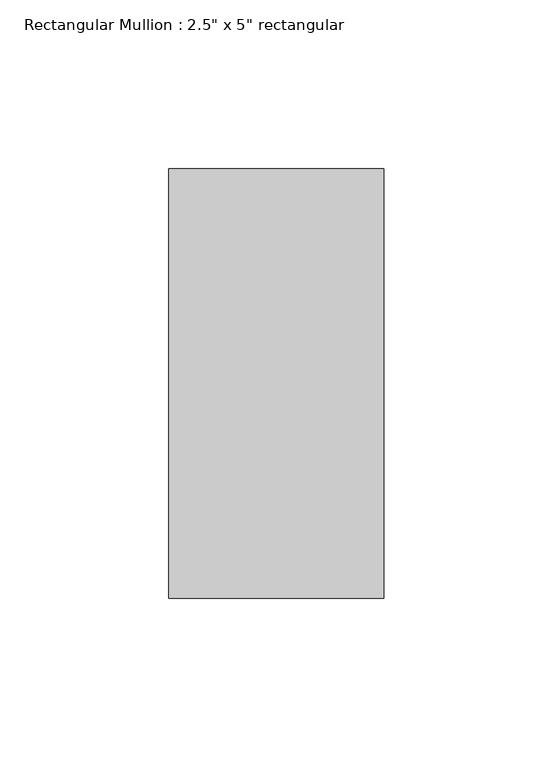
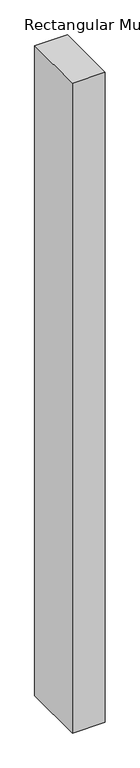
"""IFC4 building model written with IfcOpenShell, lengths in millimetres: member geometry."""

from ifc_helpers import new_model, si_unit, frame, origin, place, context, project, spatial, polyline, outline, extrude, source, transform, mapped, element, save


def member_1c68d6bd(model_context):
    return source(origin(), model_context, "Body", "SweptSolid", [
        extrude(outline(polyline([(0.0, 63.5), (0.0, -63.5), (-63.5, -63.5), (-63.5, 63.5), (0.0, 63.5)])), frame((0.0, 0.0, -1334.3185135), z_axis=(0.0, 0.0, 1.0), x_axis=(1.0, 0.0, 0.0)), (0.0, 0.0, 1.0), 1334.3185135),
    ])


if __name__ == "__main__":
    model = new_model("IFC4")
    model_context = context("Model", 3, world=origin())
    ifc_project = project(units=[si_unit("LENGTHUNIT", "METRE", prefix="MILLI")], contexts=[model_context])
    site = spatial("IfcSite", under=ifc_project)
    building = spatial("IfcBuilding", under=site)
    placement = place(None, origin())
    member_shape = member_1c68d6bd(model_context)
    element("IfcMember", 1, ObjectType="Rectangular Mullion : 2.5\" x 5\" rectangular", at=placement, inside=building, context=model_context, shape_type="MappedRepresentation", body=[
        mapped(member_shape, transform((0.0, 0.0, 0.0), x_axis=(1.0, 0.0, 0.0), y_axis=(0.0, 1.0, 0.0), z_axis=(0.0, 0.0, 1.0))),
    ])
    save(model, "model.ifc")

# Revit data of these elements
# Type "Rectangular Mullion : 2.5\" x 5\" rectangular"
#   built-in parameter 1007304 = 0.416667 (stored number, unit not read)
#   built-in parameter 1007301 = 0.104167 (stored number, unit not read)
#   built-in parameter 1007300 = 0.104167 (stored number, unit not read)
# Element 1 (IfcMember, "Rectangular Mullion : 2.5\" x 5\" rectangular")
#   Materials on its faces: "Aluminum"
# Materials
#   "Aluminum": class "Metal", colour RGB 247 247 247, transparency 0, Description = "Aluminum 6061", Cost = 0
